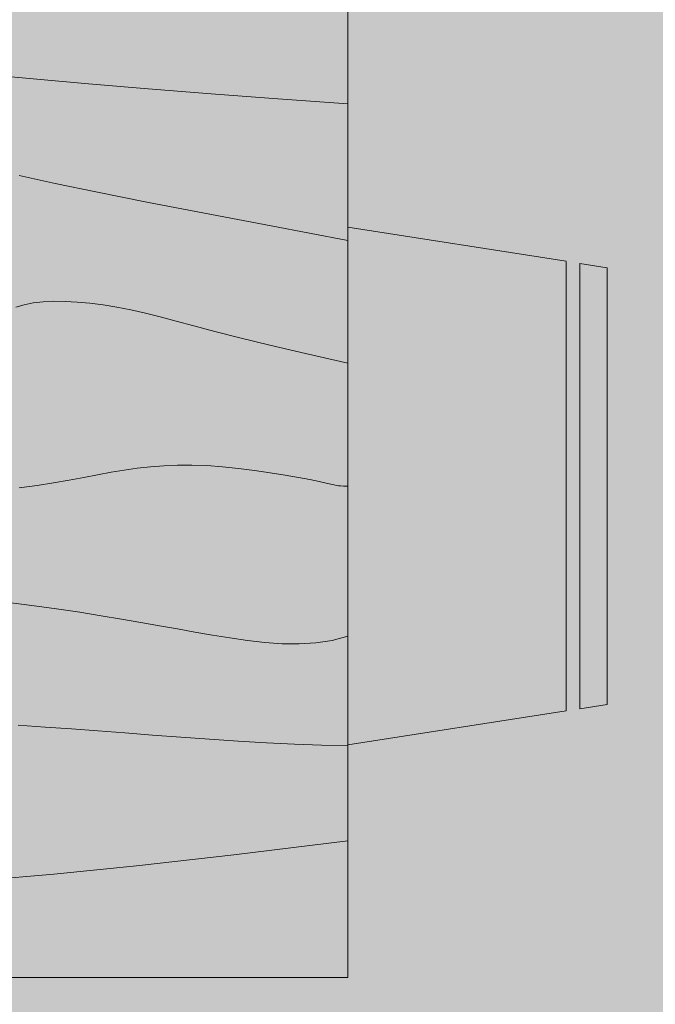
# Model space of a CAD drawing. Units: inches. Extents: x 3024 to 3952, y 1308 to 1863.
# Tile 11 of 29: x 3374 to 3392, y 1587 to 1613. Entities that reach past the tile are written whole.
import ezdxf

# ---------------------------------------------------------------- set-up
doc = ezdxf.new("R2010")
doc.units = ezdxf.units.IN
doc.layers.add('A-FLOR-PATT', color=254, linetype='Continuous', lineweight=13, true_color=0xfeeab9)
for name, color, linetype, lineweight in [('A-FLOR-TILE-PATT', 7, 'Continuous', 13), ('A-FURN', 8, 'Continuous', 18), ('A-FURN-PATT', 9, 'Continuous', 13)]:
    doc.layers.add(name, color=color, linetype=linetype, lineweight=lineweight)

# ---------------------------------------------------------------- blocks, each defined once
blk = doc.blocks.new('Dining Set - 36 x 72 in.')
for p, q in [((36, -18), (36, 18)), ((44.0006, 8.23428), (35.9976, 9.48474)), ((44, 8.23041), (44, -8.23915)), ((44.5, -8.15843), (44.5, 8.15338)), ((45.5, 8), (44.5005, 8.15617)), ((45.5, 8), (45.5, -8)), ((35.9976, -9.48476), (43.9993, -8.2345)), ((44.4997, -8.15631), (45.5, -8)), ((-36, -18), (36, -18))]:
    blk.add_line(p, q)
for points in [[(22.5879, 15.08984), (24.4721, 14.91715), (26.5052, 14.73958), (28.6809, 14.5581), (30.9929, 14.3737), (33.4347, 14.18733), (36, 14)], [(23.959, 11.37304), (25.2786, 11.08618), (26.8282, 10.76562), (28.6414, 10.40405), (30.752, 9.99414), (33.1936, 9.52856), (36, 9)], [(23.8358, 6.55957), (24.142, 6.64323), (24.4735, 6.70735), (24.8334, 6.75), (25.2235, 6.76969), (25.642, 6.76692), (26.0858, 6.74267), (26.5521, 6.69791), (27.0379, 6.63362), (27.5404, 6.55078), (28.0565, 6.45036), (28.5834, 6.33333), (29.1242, 6.19987), (29.7071, 6.04687), (30.3661, 5.87044), (31.1354, 5.66666), (32.0493, 5.43164), (33.142, 5.16146), (34.4475, 4.85221), (36, 4.5)], [(23.9549, -0.06836), (24.6146, 0.02083), (25.2235, 0.11784), (25.7904, 0.21875), (26.3241, 0.31966), (26.8334, 0.41666), (27.3265, 0.50618), (27.8099, 0.58593), (28.2894, 0.65397), (28.7709, 0.70833), (29.2601, 0.74707), (29.763, 0.76823), (30.2855, 0.76985), (30.8334, 0.75), (31.4088, 0.70784), (31.9994, 0.64713), (32.589, 0.57275), (33.1615, 0.48958), (33.7008, 0.4025), (34.1908, 0.3164), (34.6153, 0.23616), (34.9584, 0.16666), (35.2099, 0.11165), (35.3848, 0.07031), (35.504, 0.04069), (35.5886, 0.02083), (35.6594, 0.00879), (35.7377, 0.0026), (35.8442, 0.00032), (36, 0)], [(23.4727, -4.25391), (24.4289, -4.37549), (25.3334, -4.5), (26.1785, -4.62492), (26.9694, -4.74935), (27.7145, -4.87281), (28.4219, -4.99479), (29.1, -5.11483), (29.7572, -5.23242), (30.4016, -5.34709), (31.0417, -5.45834), (31.6837, -5.56437), (32.3262, -5.65821), (32.9658, -5.73153), (33.599, -5.77604), (34.2224, -5.78345), (34.8327, -5.74545), (35.4264, -5.65373), (36, -5.5)], [(23.9271, -8.76563), (24.9081, -8.82707), (25.8763, -8.89388), (26.8465, -8.96558), (27.8334, -9.04167), (28.8474, -9.12118), (29.8828, -9.20117), (30.93, -9.27824), (31.9792, -9.34896), (33.0205, -9.40991), (34.0443, -9.45768), (35.0407, -9.48885), (36, -9.5)], [(0.2448, -14.26042), (1.7647, -14.3169), (3.1973, -14.3763), (4.5507, -14.43767), (5.8333, -14.5), (7.0554, -14.5621), (8.235, -14.62175), (9.3922, -14.67652), (10.5469, -14.72396), (11.7192, -14.76164), (12.929, -14.78711), (14.1965, -14.79794), (15.5417, -14.79167), (16.9933, -14.76424), (18.6152, -14.70508), (20.4804, -14.60197), (22.6615, -14.44271), (25.2312, -14.21509), (28.2624, -13.9069), (31.8277, -13.50594), (36, -13)]]:
    blk.add_lwpolyline(points)

msp = doc.modelspace()

# ---------------------------------------------------------------- hatches: boundary and pattern name
at = {"layer": 'A-FLOR-PATT', "transparency": 33554528}
h = msp.add_hatch(color=256, dxfattribs=at)
h.dxf.hatch_style = 1
h.paths.add_polyline_path([(3460.764, 1688.6064), (3412.764, 1688.6064), (3412.764, 1694.6064), (3460.764, 1694.6064), (3460.764, 1778.6064), (3406.764, 1778.6064), (3406.764, 1759.9514), (3318.2981, 1759.9514), (3318.2981, 1658.6064), (3322.5356, 1658.6064), (3322.5356, 1652.6064), (3292.764, 1652.6064), (3292.764, 1778.6064), (3106.764, 1778.6064), (3106.764, 1628.6064), (3172.764, 1628.6064), (3172.764, 1532.6064), (3166.764, 1532.6064), (3166.764, 1628.6064), (3106.764, 1628.6064), (3106.764, 1356.8452), (3202.812, 1356.8452), (3202.812, 1354.2534), (3202.812, 1353.8388), (3202.812, 1351.1212), (3202.812, 1347.8452), (3277.764, 1347.8452), (3277.764, 1353.8452), (3277.764, 1356.8452), (3277.764, 1442.6064), (3460.764, 1442.6064)])
h.paths.add_polyline_path([(3216.238, 1527.2064), (3216.238, 1491.2064), (3214.663, 1491.2064), (3214.663, 1491.2409, -0.3966224), (3180.243, 1526.6064), (3163.0285, 1526.6064), (3163.0285, 1531.1064), (3161.716, 1531.1064), (3161.716, 1561.1064), (3163.0285, 1561.1064), (3163.0285, 1531.1064), (3163.0285, 1526.6064), (3180.243, 1526.6064, 0.3966224), (3214.663, 1491.2409), (3214.663, 1527.2064)], flags=16)
h.paths.add_polyline_path([(3227.364, 1649.8972), (3191.364, 1649.8972), (3191.364, 1651.4722), (3227.364, 1651.4722)], flags=16)
h.paths.add_polyline_path([(3323.1172, 1606.7362), (3323.8545, 1606.8514), (3323.8545, 1594.8241), (3323.1172, 1594.9393)], flags=16)
h.paths.add_polyline_path([(3324.2232, 1606.909), (3330.1216, 1607.8307), (3330.1216, 1614.1093), (3339.3495, 1614.1093), (3340.2711, 1620.0078), (3352.4136, 1620.0078), (3353.3353, 1614.1093), (3359.9941, 1614.1093), (3360.9157, 1620.0078), (3373.0582, 1620.0078), (3373.9799, 1614.1093), (3383.2077, 1614.1093), (3383.2077, 1607.8307), (3389.1062, 1606.909), (3389.1062, 1594.7665), (3383.2077, 1593.8449), (3383.2077, 1587.5663), (3373.9799, 1587.5663), (3373.0583, 1581.6678), (3360.9157, 1581.6678), (3359.9941, 1587.5663), (3353.3353, 1587.5663), (3352.4136, 1581.6678), (3340.2711, 1581.6678), (3339.3495, 1587.5663), (3330.1216, 1587.5663), (3330.1216, 1593.8449), (3324.2232, 1594.7665)], flags=16)
h.paths.add_polyline_path([(3236.1584, 1693.1064), (3236.1584, 1723.1064), (3237.4709, 1723.1064), (3237.4709, 1693.1064)], flags=16)
h.paths.add_polyline_path([(3373.2158, 1600.6847), (3373.7965, 1600.7303), (3374.3268, 1600.7874), (3374.8132, 1600.8531), (3375.2621, 1600.9247), (3375.6801, 1600.9991), (3376.0736, 1601.0735), (3376.6855, 1601.19), (3377.366, 1601.3023), (3378.0667, 1601.3814), (3378.8026, 1601.4123), (3379.5865, 1601.3839), (3380.4537, 1601.2948), (3381.301, 1601.1717), (3382.0317, 1601.0433), (3382.4398, 1600.9607), (3382.6252, 1600.9201), (3382.919, 1600.8507), (3382.9044, 1600.8531), (3382.842, 1600.8678), (3382.7541, 1600.8896), (3382.6252, 1600.9201), (3382.4398, 1600.9607), (3382.1868, 1601.0119), (3381.8738, 1601.0711), (3381.5125, 1601.1346), (3381.1149, 1601.1988), (3380.6928, 1601.2601), (3380.2581, 1601.3149), (3379.8226, 1601.3597), (3379.3984, 1601.3908), (3378.9944, 1601.4054), (3378.6092, 1601.4042), (3378.2384, 1601.3886), (3377.8777, 1601.36), (3377.5227, 1601.32), (3377.1691, 1601.2698), (3376.8127, 1601.211), (3376.4491, 1601.145), (3376.0736, 1601.0735), (3375.4177, 1600.9494), (3374.5542, 1600.8119), (3373.5044, 1600.6988)], flags=0)
h.paths.add_polyline_path([(3380.0253, 1596.7351), (3380.499, 1596.6659), (3380.9706, 1596.6119), (3381.4375, 1596.5791), (3381.8971, 1596.5736), (3382.5886, 1596.6167), (3382.7848, 1596.6692), (3382.1465, 1596.5706), (3381.236, 1596.5815), (3380.3199, 1596.6865)], flags=0)
h.paths.add_polyline_path([(3369.6414, 1603.9617), (3370.1589, 1604.0021), (3370.6218, 1604.0539), (3371.0335, 1604.1173), (3371.3978, 1604.1921), (3371.7181, 1604.2785), (3371.9984, 1604.3761), (3372.2441, 1604.483), (3372.4611, 1604.5972), (3372.655, 1604.7163), (3372.8317, 1604.8384), (3372.9968, 1604.9611), (3373.3703, 1605.2455), (3373.8426, 1605.5328), (3374.4624, 1605.7539), (3375.1058, 1605.8302), (3375.7221, 1605.8261), (3376.4109, 1605.76), (3377.1534, 1605.6376), (3377.8945, 1605.473), (3378.1382, 1605.409), (3377.7394, 1605.5074), (3377.3509, 1605.5937), (3376.9704, 1605.6677), (3376.5999, 1605.7288), (3376.2417, 1605.7762), (3375.8979, 1605.8092), (3375.5707, 1605.8271), (3375.2621, 1605.8291), (3374.9745, 1605.8146), (3374.7092, 1605.7832), (3374.4647, 1605.7359), (3374.239, 1605.6742), (3374.0298, 1605.5996), (3373.835, 1605.5134), (3373.6525, 1605.4171), (3373.4801, 1605.3123), (3373.3156, 1605.2002), (3373.1562, 1605.0825), (3372.7603, 1604.781), (3372.236, 1604.4588), (3371.5738, 1604.2283), (3370.8493, 1604.0794), (3369.9262, 1603.976)], flags=0)
h.paths.add_polyline_path([(3366.7533, 1606.5832), (3367.1713, 1606.5519), (3367.5378, 1606.5374), (3367.8568, 1606.5394), (3368.1325, 1606.5573), (3368.3694, 1606.5903), (3368.5717, 1606.6377), (3368.7438, 1606.6988), (3368.89, 1606.7728), (3369.0146, 1606.8591), (3369.121, 1606.9568), (3369.2094, 1607.0646), (3369.2792, 1607.181), (3369.3295, 1607.3046), (3369.3596, 1607.4339), (3369.3688, 1607.5676), (3369.3565, 1607.7042), (3369.3218, 1607.8422), (3369.2649, 1607.9804), (3369.1893, 1608.1187), (3369.0993, 1608.2569), (3368.9992, 1608.3952), (3368.8934, 1608.5334), (3368.7861, 1608.6717), (3368.6817, 1608.8099), (3368.4212, 1609.1804), (3368.2685, 1609.7106), (3368.4883, 1610.1814), (3369.0537, 1610.4604), (3369.6717, 1610.5097), (3370.2812, 1610.3612), (3370.4805, 1610.2968), (3370.1882, 1610.3839), (3369.9284, 1610.4472), (3369.6905, 1610.4842), (3369.4662, 1610.4933), (3369.2555, 1610.4765), (3369.0608, 1610.4367), (3368.884, 1610.3767), (3368.7274, 1610.2994), (3368.5931, 1610.2077), (3368.4833, 1610.1045), (3368.4002, 1609.9927), (3368.3451, 1609.8747), (3368.3166, 1609.7517), (3368.3127, 1609.6244), (3368.331, 1609.4935), (3368.3696, 1609.3597), (3368.4261, 1609.2237), (3368.4985, 1609.0863), (3368.5845, 1608.9482), (3368.6817, 1608.8099), (3368.7861, 1608.6717), (3368.8934, 1608.5334), (3368.9992, 1608.3952), (3369.0993, 1608.2569), (3369.3398, 1607.8876), (3369.3941, 1607.2896), (3368.9774, 1606.7817), (3368.3928, 1606.5742), (3367.7162, 1606.5303), (3367.0044, 1606.5585)], flags=0)
h.paths.add_polyline_path([(3362.1859, 1610.2589), (3362.5478, 1610.2845), (3362.8348, 1610.3275), (3363.0585, 1610.3863), (3363.2303, 1610.4595), (3363.3619, 1610.5457), (3363.463, 1610.6432), (3363.5376, 1610.7502), (3363.5876, 1610.8643), (3363.6153, 1610.9834), (3363.6229, 1611.1055), (3363.6125, 1611.2283), (3363.5861, 1611.3496), (3363.5462, 1611.4673), (3363.4949, 1611.5797), (3363.4358, 1611.6871), (3363.3723, 1611.7902), (3363.3081, 1611.8897), (3363.2468, 1611.9863), (3363.192, 1612.0808), (3363.0258, 1612.4261), (3363.3371, 1612.8672), (3363.9008, 1612.9782), (3364.4822, 1612.9641), (3365.1098, 1612.9074), (3365.328, 1612.8805), (3364.9615, 1612.9208), (3364.6426, 1612.9496), (3364.3668, 1612.9669), (3364.1299, 1612.9726), (3363.9276, 1612.9669), (3363.7555, 1612.9496), (3363.6093, 1612.9208), (3363.4848, 1612.8805), (3363.3782, 1612.8289), (3363.2889, 1612.7672), (3363.2169, 1612.6969), (3363.1622, 1612.6193), (3363.1247, 1612.5361), (3363.1046, 1612.4484), (3363.1017, 1612.358), (3363.1161, 1612.266), (3363.1472, 1612.1738), (3363.192, 1612.0808), (3363.2468, 1611.9863), (3363.3081, 1611.8897), (3363.3723, 1611.7902), (3363.4358, 1611.6871), (3363.6363, 1611.323), (3363.5979, 1610.7003), (3363.0863, 1610.3651), (3362.3983, 1610.2622)], flags=0)
h.paths.add_polyline_path([(3352.356, 1581.2991), (3352.2408, 1580.5618), (3340.4439, 1580.5618), (3340.3287, 1581.2991)], flags=16)
h.paths.add_polyline_path([(3340.4439, 1621.1137), (3352.2408, 1621.1137), (3352.356, 1620.3764), (3340.3287, 1620.3764)], flags=16)
h.paths.add_polyline_path([(3278.4282, 1504.7424), (3290.3831, 1504.7424), (3290.3831, 1502.7499), (3291.0473, 1502.7499), (3291.0473, 1494.7799), (3290.3831, 1494.7799), (3290.3831, 1494.1158), (3291.0473, 1494.1158), (3291.0473, 1486.1458), (3290.3831, 1486.1458), (3290.3831, 1484.1533), (3291.0473, 1484.1533), (3291.0473, 1483.4892, -0.0909091), (3291.0473, 1468.8776), (3291.0473, 1468.2135), (3290.3831, 1468.2135), (3290.3831, 1464.8926), (3278.4282, 1464.8926), (3278.4282, 1472.8626), (3277.764, 1473.5268), (3277.764, 1478.84), (3278.4282, 1479.5042)], flags=16)
h.paths.add_polyline_path([(3278.7603, 1504.4103), (3290.051, 1504.4103), (3290.051, 1465.2247), (3278.7603, 1465.2247)], flags=0)
h.paths.add_polyline_path([(3123.904, 1600.7821), (3117.9039, 1602.7821), (3117.9039, 1599.7821), (3119.4039, 1599.7821), (3119.4039, 1596.7821), (3118.4039, 1596.7821), (3118.4039, 1598.7821), (3117.9039, 1598.7821), (3117.9039, 1596.2821), (3109.9039, 1596.2821), (3109.9039, 1617.2821), (3117.9039, 1617.2821), (3117.9039, 1610.7821), (3123.9038, 1612.7821, -0.7025712), (3137.9039, 1606.7822, -0.7025621)], flags=16)
h.paths.add_polyline_path([(3123.9039, 1602.7822), (3123.9039, 1610.7822, -0.7345333), (3136.9039, 1606.7822, -0.7345297)], flags=0)
h.paths.add_polyline_path([(3177.972, 1689.6473), (3109.2405, 1689.6473), (3109.2405, 1741.1959), (3177.972, 1741.1959)], flags=16)
h.paths.add_polyline_path([(3373.0006, 1581.2991), (3372.8854, 1580.5618), (3361.0885, 1580.5618), (3360.9733, 1581.2991)], flags=16)
h.paths.add_polyline_path([(3361.0885, 1621.1137), (3372.8854, 1621.1137), (3373.0006, 1620.3764), (3360.9733, 1620.3764)], flags=16)
h.paths.add_polyline_path([(3116.9039, 1598.2821, -0.4142136), (3116.1539, 1597.2821), (3111.9039, 1597.2821, -0.4142136), (3110.9039, 1598.0321), (3110.9039, 1615.2821, -0.4142136), (3111.6539, 1616.2821), (3115.9039, 1616.2821, -0.4142136), (3116.9039, 1615.5321)], flags=0)
h.paths.add_polyline_path([(3121.6122, 1728.1369), (3121.6122, 1696.5205), (3110.2715, 1696.5205), (3110.2715, 1714.3906), (3121.6122, 1714.3906), (3121.6122, 1716.4526), (3110.2715, 1716.4526), (3110.2715, 1734.3228), (3123.3304, 1734.3228), (3123.3304, 1729.8552), (3134.6711, 1741.1959), (3134.6711, 1728.1369)], flags=0)
h.paths.add_polyline_path([(3389.4748, 1606.8514), (3390.2122, 1606.7362), (3390.2122, 1594.9393), (3389.4748, 1594.8241)], flags=16)
h.paths.add_polyline_path([(3257.6842, 1762.8281), (3259.6842, 1768.8281), (3256.6842, 1768.8281), (3256.6842, 1767.3281), (3253.6842, 1767.3281), (3253.6842, 1768.3281), (3255.6842, 1768.3281), (3255.6842, 1768.8281), (3253.1842, 1768.8281), (3253.1842, 1776.8281), (3274.1842, 1776.8281), (3274.1842, 1768.8281), (3267.6842, 1768.8281), (3269.6842, 1762.8282, -0.7025712), (3263.6843, 1748.8282, -0.7025621)], flags=16)
h.paths.add_polyline_path([(3259.6842, 1762.8281), (3267.6843, 1762.8281, -0.7345333), (3263.6842, 1749.8282, -0.7345297)], flags=0)
h.paths.add_polyline_path([(3411.264, 1715.6064), (3411.264, 1716.9189), (3441.264, 1716.9189), (3441.264, 1715.6064)], flags=16)
h.paths.add_polyline_path([(3178.3806, 1449.1876), (3178.3806, 1397.639), (3109.6491, 1397.639), (3109.6491, 1449.1876)], flags=16)
h.paths.add_polyline_path([(3397.1501, 1541.7146), (3419.6183, 1541.7146), (3419.6183, 1496.7783), (3397.1501, 1496.7783)], flags=16)
h.paths.add_polyline_path([(3254.1842, 1770.5781), (3254.1842, 1774.8281, -0.4142136), (3254.9342, 1775.8281), (3272.1842, 1775.8281, -0.4142136), (3273.1842, 1775.0781), (3273.1842, 1770.8281, -0.4142136), (3272.4342, 1769.8281), (3255.1842, 1769.8281, -0.4142136)], flags=0)
h.paths.add_polyline_path([(3403.672, 1500.7601), (3403.6016, 1500.3997), (3403.5328, 1500.0441), (3403.4662, 1499.6867), (3403.4027, 1499.3226), (3403.3464, 1498.9532), (3403.3025, 1498.5811), (3403.2759, 1498.2091), (3403.2714, 1497.8401), (3403.3064, 1497.2813), (3403.3491, 1497.1219), (3403.2689, 1497.6395), (3403.2778, 1498.3719), (3403.3635, 1499.0984), (3403.4889, 1499.8168), (3403.6016, 1500.3997), (3403.672, 1500.7601), (3403.744, 1501.1315), (3403.817, 1501.5205), (3403.891, 1501.9336), (3403.9656, 1502.3769), (3404.0404, 1502.8572), (3404.115, 1503.3786), (3404.2264, 1504.2311), (3404.2571, 1504.5223), (3404.1552, 1503.6598), (3404.0063, 1502.6193), (3403.8604, 1501.7518), (3403.744, 1501.1315)], flags=0)
h.paths.add_polyline_path([(3406.5868, 1505.0416), (3406.6121, 1504.5236), (3406.6492, 1504.0526), (3406.6956, 1503.624), (3406.7491, 1503.2333), (3406.8072, 1502.8759), (3406.8676, 1502.5473), (3406.9281, 1502.243), (3407.0268, 1501.7597), (3407.1416, 1501.1368), (3407.2087, 1500.3904), (3407.1804, 1499.6703), (3407.1078, 1498.9956), (3407.0074, 1498.3199), (3406.8809, 1497.6059), (3406.7403, 1496.9627), (3406.7418, 1496.9824), (3406.7491, 1497.0249), (3406.8229, 1497.3409), (3406.8364, 1497.4025), (3406.878, 1497.6078), (3406.9261, 1497.8614), (3406.9777, 1498.1526), (3407.0298, 1498.4712), (3407.0797, 1498.8068), (3407.1243, 1499.149), (3407.1607, 1499.4874), (3407.1859, 1499.8115), (3407.1978, 1500.1137), (3407.1969, 1500.3962), (3407.1841, 1500.6642), (3407.1609, 1500.9225), (3407.1284, 1501.1761), (3407.0876, 1501.43), (3407.0398, 1501.6891), (3406.9862, 1501.9585), (3406.8832, 1502.4628), (3406.7712, 1503.0713), (3406.6657, 1503.8424), (3406.5924, 1504.7735)], flags=0)
h.paths.add_polyline_path([(3409.2517, 1507.8962), (3409.2752, 1507.4282), (3409.3079, 1507.0076), (3409.3501, 1506.6314), (3409.4015, 1506.2969), (3409.4624, 1506.0009), (3409.5326, 1505.7406), (3409.6119, 1505.5128), (3409.6988, 1505.3131), (3409.7915, 1505.1368), (3409.8883, 1504.9792), (3409.9875, 1504.8356), (3410.0872, 1504.7015), (3410.1859, 1504.572), (3410.4508, 1504.2132), (3410.7205, 1503.6035), (3410.8059, 1502.8824), (3410.7619, 1502.0875), (3410.6122, 1501.2299), (3410.4402, 1500.6169), (3410.2538, 1500.0031), (3410.0536, 1499.3219), (3409.9909, 1499.0812), (3410.1761, 1499.7472), (3410.3596, 1500.3513), (3410.4512, 1500.6561), (3410.5312, 1500.9412), (3410.6013, 1501.226), (3410.6614, 1501.512), (3410.7111, 1501.7964), (3410.7496, 1502.0763), (3410.7764, 1502.3489), (3410.7909, 1502.6114), (3410.7926, 1502.8608), (3410.7808, 1503.0944), (3410.7553, 1503.31), (3410.7169, 1503.5087), (3410.6667, 1503.6921), (3410.6061, 1503.8621), (3410.5361, 1504.0203), (3410.4578, 1504.1686), (3410.3726, 1504.3088), (3410.2815, 1504.4424), (3410.1859, 1504.572), (3410.0872, 1504.7015), (3409.859, 1505.0083), (3409.5943, 1505.5117), (3409.4266, 1506.1336), (3409.324, 1506.8011), (3409.2586, 1507.6407)], flags=0)
h.paths.add_polyline_path([(3411.4914, 1510.5878), (3411.4432, 1510.1586), (3411.4054, 1509.775), (3411.38, 1509.4354), (3411.3681, 1509.1376), (3411.3698, 1508.8784), (3411.3843, 1508.6542), (3411.4112, 1508.4618), (3411.4497, 1508.2974), (3411.4994, 1508.1575), (3411.5595, 1508.0388), (3411.6296, 1507.9375), (3411.7097, 1507.851), (3411.802, 1507.7792), (3411.9096, 1507.7225), (3412.0353, 1507.6817), (3412.1821, 1507.6572), (3412.3528, 1507.6496), (3412.5505, 1507.6597), (3412.778, 1507.6879), (3413.0364, 1507.7341), (3413.3194, 1507.7955), (3413.6188, 1507.8687), (3413.9264, 1507.95), (3414.234, 1508.036), (3414.5333, 1508.1232), (3414.8163, 1508.208), (3415.0747, 1508.287), (3415.3023, 1508.3569), (3415.5007, 1508.4158), (3415.6733, 1508.4617), (3416.1158, 1508.5538), (3416.512, 1508.2591), (3416.716, 1507.6581), (3416.61, 1507.0003), (3416.3052, 1506.3411), (3415.8928, 1505.618), (3415.7339, 1505.3633), (3415.9914, 1505.791), (3416.201, 1506.1583), (3416.3666, 1506.4739), (3416.4925, 1506.7462), (3416.5828, 1506.9838), (3416.6413, 1507.1949), (3416.6725, 1507.3883), (3416.6799, 1507.5705), (3416.6662, 1507.7417), (3416.6339, 1507.9), (3416.5851, 1508.0436), (3416.5223, 1508.1709), (3416.4478, 1508.28), (3416.3639, 1508.3692), (3416.273, 1508.4368), (3416.1765, 1508.4815), (3416.0718, 1508.5047), (3415.9553, 1508.5079), (3415.8237, 1508.493), (3415.6733, 1508.4617), (3415.5007, 1508.4158), (3415.3327, 1508.3659), (3414.6495, 1508.157), (3414.0606, 1507.9855), (3413.4456, 1507.8229), (3412.8838, 1507.701), (3412.5505, 1507.6597), (3412.0748, 1507.6354), (3411.595, 1507.8883), (3411.398, 1508.4429), (3411.3624, 1508.9927), (3411.3854, 1509.5711), (3411.4578, 1510.3071)], flags=0)
h.paths.add_polyline_path([(3135.0797, 1449.1876), (3135.0797, 1436.1286), (3122.0208, 1436.1286), (3122.0208, 1404.5122), (3110.6801, 1404.5122), (3110.6801, 1422.3823), (3122.0208, 1422.3823), (3122.0208, 1424.4443), (3110.6801, 1424.4443), (3110.6801, 1442.3145), (3123.739, 1442.3145), (3123.739, 1437.8469)], flags=0)
h.paths.add_polyline_path([(3416.4944, 1514.2949), (3416.4837, 1513.8511), (3416.4893, 1513.4867), (3416.5102, 1513.1926), (3416.5451, 1512.9593), (3416.5929, 1512.7775), (3416.6524, 1512.6379), (3416.7224, 1512.531), (3416.8017, 1512.4488), (3416.8886, 1512.3882), (3416.9813, 1512.3476), (3417.0781, 1512.3251), (3417.1773, 1512.3189), (3417.277, 1512.3274), (3417.3757, 1512.3488), (3417.4713, 1512.3813), (3417.5627, 1512.4229), (3417.65, 1512.471), (3417.7338, 1512.5225), (3417.8146, 1512.5747), (3417.8931, 1512.6245), (3417.9699, 1512.6691), (3418.2968, 1512.8265), (3418.6505, 1512.4645), (3418.7037, 1511.9342), (3418.6693, 1511.3839), (3418.6076, 1510.8228), (3418.5777, 1510.5927), (3418.6197, 1510.9333), (3418.6525, 1511.2311), (3418.6759, 1511.4903), (3418.6899, 1511.7144), (3418.6946, 1511.9069), (3418.6899, 1512.0713), (3418.6759, 1512.2112), (3418.6525, 1512.33), (3418.6197, 1512.4311), (3418.5778, 1512.5177), (3418.5276, 1512.5903), (3418.4705, 1512.6488), (3418.4075, 1512.6933), (3418.3399, 1512.7237), (3418.2686, 1512.7401), (3418.1951, 1512.7424), (3418.1204, 1512.7307), (3418.0455, 1512.7055), (3417.9792, 1512.6736), (3417.65, 1512.471), (3417.5627, 1512.4229), (3417.4713, 1512.3813), (3417.3757, 1512.3488), (3417.277, 1512.3274), (3416.878, 1512.2936), (3416.5757, 1512.7549), (3416.492, 1513.3145), (3416.4808, 1514.0384)], flags=0)
h.paths.add_polyline_path([(3392.8223, 1481.9454), (3396.7707, 1481.9454), (3396.7707, 1480.9201), (3428.3585, 1480.9201), (3428.3585, 1481.9454), (3432.3069, 1481.9454), (3432.3069, 1464.8354, -0.266667), (3392.8223, 1464.8354)], flags=16)
h.paths.add_polyline_path([(3431.203, 1547.5428), (3450.8613, 1547.5428, -0.1904762), (3450.8614, 1484.031), (3431.203, 1484.031), (3431.203, 1488.5675), (3432.3809, 1488.5675), (3432.3809, 1543.0062), (3431.203, 1543.0062)], flags=16)
h.paths.add_polyline_path([(3451.9233, 1524.86, -0.0496282), (3451.9233, 1506.7138), (3446.7921, 1506.7138), (3446.7921, 1524.86)], flags=0)
h.paths.add_polyline_path([(3460.764, 1436.6064), (3277.764, 1436.6064), (3277.764, 1356.8452), (3277.764, 1353.8452), (3460.764, 1353.8452)], flags=17)
h.paths.add_polyline_path([(3121.3033, 1577.378), (3153.693, 1577.378), (3153.693, 1586.6752), (3121.3033, 1586.6752)], flags=24)
h.paths.add_polyline_path([(3164.1457, 1464.1276), (3210.4801, 1464.1276), (3210.4801, 1473.4247), (3164.1457, 1473.4247)], flags=24)
h.paths.add_polyline_path([(3343.1909, 1505.8863), (3373.7236, 1505.8863), (3373.7236, 1515.1773), (3343.1909, 1515.1773)], flags=24)
h.paths.add_polyline_path([(3337.6353, 1564.2926), (3370.0189, 1564.2926), (3370.0189, 1573.5836), (3337.6353, 1573.5836)], flags=24)
h.paths.add_polyline_path([(3419.204, 1753.8578), (3453.3997, 1753.8578), (3453.3997, 1762.9956), (3419.204, 1762.9956)], flags=24)
h.paths.add_polyline_path([(3341.2523, 1701.0246), (3381.0761, 1701.0246), (3381.0761, 1710.3156), (3341.2523, 1710.3156)], flags=24)
h.paths.add_polyline_path([(3245.8895, 1726.2997), (3278.2793, 1726.2997), (3278.2793, 1735.5968), (3245.8895, 1735.5968)], flags=24)
h.paths.add_polyline_path([(3128.8045, 1668.6736), (3175.1389, 1668.6736), (3175.1389, 1677.9707), (3128.8045, 1677.9707)], flags=24)
h.paths.add_polyline_path([(3345.9997, 1396.0062), (3389.09, 1396.0062), (3389.09, 1405.3033), (3345.9997, 1405.3033)], flags=24)
at = {"layer": 'A-FLOR-TILE-PATT', "transparency": 33554569}
h = msp.add_hatch(dxfattribs=at)
h.set_pattern_fill('ANGLE', color=256, scale=2)
h.set_pattern_definition([(0, (0, 0), (0, 13.97), [10.16, -3.81]), (90, (0, 0), (-13.97, 9e-16), [10.16, -3.81])])
h.paths.add_polyline_path([(3292.764, 1778.6064), (3232.764, 1778.6064), (3232.764, 1694.6064), (3236.1584, 1694.6064), (3236.1584, 1723.1064), (3237.4709, 1723.1064), (3237.4709, 1723.0777, -0.3870039), (3266.1209, 1694.6064), (3292.764, 1694.6064)])
h.paths.add_polyline_path([(3263.6843, 1748.8282, -0.7025621), (3257.6842, 1762.8281), (3259.6842, 1768.8281), (3256.6842, 1768.8281), (3256.6842, 1767.3281), (3253.6842, 1767.3281), (3253.6842, 1768.3281), (3255.6842, 1768.3281), (3255.6842, 1768.8281), (3253.1842, 1768.8281), (3253.1842, 1776.8281), (3274.1842, 1776.8281), (3274.1842, 1768.8281), (3267.6842, 1768.8281), (3269.6842, 1762.8282, -0.7025712)], flags=16)
h.paths.add_polyline_path([(3263.6842, 1749.8282, -0.7345297), (3259.6842, 1762.8281), (3267.6843, 1762.8281, -0.7345333)], flags=0)
h.paths.add_polyline_path([(3255.1842, 1769.8281, -0.4142136), (3254.1842, 1770.5781), (3254.1842, 1774.8281, -0.4142136), (3254.9342, 1775.8281), (3272.1842, 1775.8281, -0.4142136), (3273.1842, 1775.0781), (3273.1842, 1770.8281, -0.4142136), (3272.4342, 1769.8281)], flags=0)
h.paths.add_polyline_path([(3460.764, 1436.6064), (3277.764, 1436.6064), (3277.764, 1356.8452), (3277.764, 1353.8452), (3460.764, 1353.8452)])
h.paths.add_polyline_path([(3166.764, 1628.6064), (3106.764, 1628.6064), (3106.764, 1532.6064), (3133.066, 1532.6064, -0.3870039), (3161.716, 1561.0777), (3161.716, 1561.1064), (3163.0285, 1561.1064), (3163.0285, 1532.6064), (3166.764, 1532.6064)])
h.paths.add_polyline_path([(3123.904, 1600.7821), (3117.9039, 1602.7821), (3117.9039, 1599.7821), (3119.4039, 1599.7821), (3119.4039, 1596.7821), (3118.4039, 1596.7821), (3118.4039, 1598.7821), (3117.9039, 1598.7821), (3117.9039, 1596.2821), (3109.9039, 1596.2821), (3109.9039, 1617.2821), (3117.9039, 1617.2821), (3117.9039, 1610.7821), (3123.9038, 1612.7821, -0.7025712), (3137.9039, 1606.7822, -0.7025621)], flags=16)
h.paths.add_polyline_path([(3123.9039, 1602.7822), (3123.9039, 1610.7822, -0.7345333), (3136.9039, 1606.7822, -0.7345297)], flags=0)
h.paths.add_polyline_path([(3116.1539, 1597.2821), (3111.9039, 1597.2821, -0.4142136), (3110.9039, 1598.0321), (3110.9039, 1615.2821, -0.4142136), (3111.6539, 1616.2821), (3115.9039, 1616.2821, -0.4142136), (3116.9039, 1615.5321), (3116.9039, 1598.2821, -0.4142136)], flags=0)
h.paths.add_polyline_path([(3245.8895, 1726.2997), (3278.2793, 1726.2997), (3278.2793, 1735.5968), (3245.8895, 1735.5968)], flags=24)
h.paths.add_polyline_path([(3345.9997, 1396.0062), (3389.09, 1396.0062), (3389.09, 1405.3033), (3345.9997, 1405.3033)], flags=24)
h.paths.add_polyline_path([(3121.3033, 1577.378), (3153.693, 1577.378), (3153.693, 1586.6752), (3121.3033, 1586.6752)], flags=24)
at = {"layer": 'A-FURN-PATT', "transparency": 33554511}
h = msp.add_hatch(color=256, dxfattribs=at)
h.dxf.hatch_style = 1
h.paths.add_polyline_path([(3373.0582, 1620.0078), (3360.9157, 1620.0078), (3359.9941, 1614.1093), (3373.9799, 1614.1093)])
h.paths.add_polyline_path([(3372.8854, 1621.1137), (3361.0885, 1621.1137), (3360.9733, 1620.3764), (3373.0006, 1620.3764)])
h.paths.add_polyline_path([(3389.1062, 1606.909), (3383.2077, 1607.8307), (3383.2077, 1593.8449), (3389.1062, 1594.7665)])
h.paths.add_polyline_path([(3390.2122, 1606.7362), (3389.4748, 1606.8514), (3389.4748, 1594.8241), (3390.2122, 1594.9393)])
h.paths.add_polyline_path([(3373.9799, 1587.5663), (3359.9941, 1587.5663), (3360.9157, 1581.6678), (3373.0583, 1581.6678)])
h.paths.add_polyline_path([(3373.0006, 1581.2991), (3360.9733, 1581.2991), (3361.0885, 1580.5618), (3372.8854, 1580.5618)])
h.paths.add_polyline_path([(3353.3353, 1587.5663), (3339.3495, 1587.5663), (3340.2711, 1581.6678), (3352.4136, 1581.6678)])
h.paths.add_polyline_path([(3352.356, 1581.2991), (3340.3287, 1581.2991), (3340.4439, 1580.5618), (3352.2408, 1580.5618)])
h.paths.add_polyline_path([(3330.1216, 1607.8307), (3324.2232, 1606.909), (3324.2232, 1594.7665), (3330.1216, 1593.8449)])
h.paths.add_polyline_path([(3323.8545, 1606.8514), (3323.1172, 1606.7362), (3323.1172, 1594.9393), (3323.8545, 1594.8241)])
h.paths.add_polyline_path([(3352.4136, 1620.0078), (3340.2711, 1620.0078), (3339.3495, 1614.1093), (3353.3353, 1614.1093)])
h.paths.add_polyline_path([(3352.2408, 1621.1137), (3340.4439, 1621.1137), (3340.3287, 1620.3764), (3352.356, 1620.3764)])
at = {"layer": 'A-FURN-PATT', "transparency": 33554600}
h = msp.add_hatch(color=256, dxfattribs=at)
h.dxf.hatch_style = 1
h.paths.add_polyline_path([(3363.5462, 1611.4673), (3363.4949, 1611.5797), (3363.4358, 1611.6871), (3363.3723, 1611.7902), (3363.2557, 1611.9708), (3363.16, 1612.1359), (3363.1003, 1612.3129), (3363.1061, 1612.4946), (3363.1815, 1612.6623), (3363.3264, 1612.8038), (3363.5397, 1612.9071), (3363.7555, 1612.9496), (3363.9276, 1612.9669), (3364.1299, 1612.9726), (3364.3668, 1612.9669), (3364.6426, 1612.9496), (3364.9615, 1612.9208), (3365.328, 1612.8805), (3365.7471, 1612.8287), (3366.2271, 1612.7662), (3366.7769, 1612.6936), (3367.4055, 1612.6117), (3368.1221, 1612.5211), (3368.9354, 1612.4225), (3369.8546, 1612.3168), (3370.8886, 1612.2046), (3372.0442, 1612.0866), (3373.3189, 1611.9636), (3374.7081, 1611.8363), (3376.2072, 1611.7054), (3377.8113, 1611.5716), (3379.516, 1611.4356), (3381.3163, 1611.2982), (3383.2077, 1611.1601), (3383.2077, 1614.1093), (3330.1216, 1614.1093), (3330.1216, 1611.8974), (3333.6775, 1611.8808), (3336.899, 1611.834), (3339.8144, 1611.7613), (3342.4523, 1611.667), (3344.8411, 1611.5554), (3347.0091, 1611.4308), (3348.985, 1611.2976), (3350.797, 1611.1601), (3352.4691, 1611.0223), (3354.0078, 1610.8874), (3355.4146, 1610.7583), (3356.6916, 1610.6378), (3357.8403, 1610.5289), (3358.8627, 1610.4343), (3359.7605, 1610.357), (3360.5355, 1610.2999), (3361.1912, 1610.2651), (3361.7375, 1610.2519), (3362.1859, 1610.2589), (3362.5478, 1610.2845), (3362.8348, 1610.3275), (3363.0585, 1610.3863), (3363.2303, 1610.4595), (3363.3619, 1610.5457), (3363.463, 1610.6432), (3363.5376, 1610.7502), (3363.5876, 1610.8643), (3363.6153, 1610.9834), (3363.6229, 1611.1055), (3363.6125, 1611.2283), (3363.5861, 1611.3496)])
h.paths.add_polyline_path([(3368.8934, 1608.5334), (3368.7093, 1608.7706), (3368.5315, 1609.0235), (3368.3879, 1609.2961), (3368.3108, 1609.5637), (3368.3187, 1609.8182), (3368.4002, 1609.9927), (3368.4833, 1610.1045), (3368.5931, 1610.2077), (3368.7274, 1610.2994), (3368.884, 1610.3767), (3369.0608, 1610.4367), (3369.2555, 1610.4765), (3369.4662, 1610.4933), (3369.6905, 1610.4842), (3369.9284, 1610.4472), (3370.1882, 1610.3839), (3370.4805, 1610.2968), (3370.8156, 1610.1885), (3371.204, 1610.0615), (3371.6561, 1609.9183), (3372.1824, 1609.7614), (3372.7933, 1609.5933), (3373.5016, 1609.4153), (3374.3298, 1609.2232), (3375.3028, 1609.0117), (3376.4453, 1608.7754), (3377.7822, 1608.5088), (3379.3383, 1608.2065), (3381.1386, 1607.8633), (3383.2077, 1607.4735), (3383.2077, 1611.1601), (3381.3163, 1611.2982), (3379.516, 1611.4356), (3377.8113, 1611.5716), (3376.2072, 1611.7054), (3374.7081, 1611.8363), (3373.3189, 1611.9636), (3372.0442, 1612.0866), (3370.8886, 1612.2046), (3369.8546, 1612.3168), (3368.9354, 1612.4225), (3368.1221, 1612.5211), (3367.4055, 1612.6117), (3366.7769, 1612.6936), (3366.2271, 1612.7662), (3365.7471, 1612.8287), (3365.328, 1612.8805), (3364.9615, 1612.9208), (3364.6426, 1612.9496), (3364.3668, 1612.9669), (3364.1299, 1612.9726), (3363.9276, 1612.9669), (3363.7555, 1612.9496), (3363.6093, 1612.9208), (3363.4848, 1612.8805), (3363.3782, 1612.8289), (3363.2889, 1612.7672), (3363.2169, 1612.6969), (3363.1622, 1612.6193), (3363.1247, 1612.5361), (3363.1046, 1612.4484), (3363.1017, 1612.358), (3363.1161, 1612.266), (3363.1472, 1612.1738), (3363.192, 1612.0808), (3363.2468, 1611.9863), (3363.3081, 1611.8897), (3363.4181, 1611.7194), (3363.529, 1611.5178), (3363.6075, 1611.2866), (3363.6284, 1611.0397), (3363.5728, 1610.8008), (3363.4229, 1610.5856), (3363.2303, 1610.4595), (3363.0585, 1610.3863), (3362.8348, 1610.3275), (3362.5478, 1610.2845), (3362.1859, 1610.2589), (3361.7375, 1610.2519), (3361.1912, 1610.2651), (3360.5355, 1610.2999), (3359.7605, 1610.357), (3358.8627, 1610.4343), (3357.8403, 1610.5289), (3356.6916, 1610.6378), (3355.4146, 1610.7583), (3354.0078, 1610.8874), (3352.4691, 1611.0223), (3350.797, 1611.1601), (3348.985, 1611.2976), (3347.0091, 1611.4308), (3344.8411, 1611.5554), (3342.4523, 1611.667), (3339.8144, 1611.7613), (3336.899, 1611.834), (3333.6775, 1611.8808), (3330.1216, 1611.8974), (3330.1216, 1608.2109), (3335.3, 1608.3161), (3339.5794, 1608.3616), (3343.0805, 1608.3567), (3345.9238, 1608.3107), (3348.23, 1608.2331), (3350.1196, 1608.1331), (3351.7134, 1608.0202), (3353.1317, 1607.9036), (3354.475, 1607.7912), (3355.7618, 1607.6838), (3356.9902, 1607.5807), (3358.1585, 1607.4812), (3359.2649, 1607.3846), (3360.3076, 1607.2902), (3361.2846, 1607.1972), (3362.1945, 1607.1049), (3363.0358, 1607.0131), (3363.8102, 1606.9234), (3364.5198, 1606.8381), (3365.1667, 1606.7593), (3365.7532, 1606.6891), (3366.2814, 1606.6297), (3366.7533, 1606.5832), (3367.1713, 1606.5519), (3367.5378, 1606.5374), (3367.8568, 1606.5394), (3368.1325, 1606.5573), (3368.3694, 1606.5903), (3368.5717, 1606.6377), (3368.7438, 1606.6988), (3368.89, 1606.7728), (3369.0146, 1606.8591), (3369.121, 1606.9568), (3369.2094, 1607.0646), (3369.2792, 1607.181), (3369.3295, 1607.3046), (3369.3596, 1607.4339), (3369.3688, 1607.5676), (3369.3565, 1607.7042), (3369.3218, 1607.8422), (3369.2649, 1607.9804), (3369.1893, 1608.1187), (3369.0993, 1608.2569), (3368.9992, 1608.3952)])
h.paths.add_polyline_path([(3374.239, 1605.6742), (3374.4647, 1605.7359), (3374.7092, 1605.7832), (3374.9745, 1605.8146), (3375.2621, 1605.8291), (3375.5707, 1605.8271), (3375.8979, 1605.8092), (3376.2417, 1605.7762), (3376.5999, 1605.7288), (3376.9704, 1605.6677), (3377.3509, 1605.5937), (3377.7394, 1605.5074), (3378.1382, 1605.409), (3378.5679, 1605.2962), (3379.0538, 1605.1661), (3379.621, 1605.0159), (3380.2949, 1604.8426), (3381.1005, 1604.6434), (3382.0631, 1604.4154), (3383.2077, 1604.1557), (3383.2077, 1607.4735), (3381.1386, 1607.8633), (3379.3383, 1608.2065), (3377.7822, 1608.5088), (3376.4453, 1608.7754), (3375.3028, 1609.0117), (3374.3298, 1609.2232), (3373.5016, 1609.4153), (3372.7933, 1609.5933), (3372.1824, 1609.7614), (3371.6561, 1609.9183), (3371.204, 1610.0615), (3370.8156, 1610.1885), (3370.4805, 1610.2968), (3370.1882, 1610.3839), (3369.9284, 1610.4472), (3369.6905, 1610.4842), (3369.4662, 1610.4933), (3369.2555, 1610.4765), (3369.0608, 1610.4367), (3368.884, 1610.3767), (3368.7274, 1610.2994), (3368.5931, 1610.2077), (3368.4833, 1610.1045), (3368.4002, 1609.9927), (3368.3451, 1609.8747), (3368.3166, 1609.7517), (3368.3127, 1609.6244), (3368.331, 1609.4935), (3368.3696, 1609.3597), (3368.4261, 1609.2237), (3368.4985, 1609.0863), (3368.5845, 1608.9482), (3368.6817, 1608.8099), (3368.7861, 1608.6717), (3368.9798, 1608.422), (3369.1584, 1608.1753), (3369.306, 1607.9053), (3369.3736, 1607.6361), (3369.355, 1607.3674), (3369.2539, 1607.1187), (3369.121, 1606.9568), (3369.0146, 1606.8591), (3368.89, 1606.7728), (3368.7438, 1606.6988), (3368.5717, 1606.6377), (3368.3694, 1606.5903), (3368.1325, 1606.5573), (3367.8568, 1606.5394), (3367.5378, 1606.5374), (3367.1713, 1606.5519), (3366.7533, 1606.5832), (3366.2814, 1606.6297), (3365.7532, 1606.6891), (3365.1667, 1606.7593), (3364.5198, 1606.8381), (3363.8102, 1606.9234), (3363.0358, 1607.0131), (3362.1945, 1607.1049), (3361.2846, 1607.1972), (3360.3076, 1607.2902), (3359.2649, 1607.3846), (3358.1585, 1607.4812), (3356.9902, 1607.5807), (3355.7618, 1607.6838), (3354.475, 1607.7912), (3353.1317, 1607.9036), (3351.7134, 1608.0202), (3350.1196, 1608.1331), (3348.23, 1608.2331), (3345.9238, 1608.3107), (3343.0805, 1608.3567), (3339.5794, 1608.3616), (3335.3, 1608.3161), (3330.1216, 1608.2109), (3330.1216, 1604.893), (3334.0178, 1604.7712), (3337.4438, 1604.6789), (3340.4479, 1604.6111), (3343.0782, 1604.5627), (3345.3832, 1604.5288), (3347.4109, 1604.5042), (3349.2096, 1604.4839), (3350.8276, 1604.4629), (3352.3079, 1604.4371), (3353.6722, 1604.4062), (3354.9372, 1604.3711), (3356.1194, 1604.3323), (3357.2353, 1604.2907), (3358.3015, 1604.2469), (3359.3347, 1604.2016), (3360.3512, 1604.1557), (3361.3635, 1604.1098), (3362.3673, 1604.0654), (3363.3537, 1604.0239), (3364.3142, 1603.9867), (3365.2402, 1603.9553), (3366.1229, 1603.931), (3366.9539, 1603.9154), (3367.7243, 1603.9099), (3368.4277, 1603.9157), (3369.0654, 1603.9329), (3369.6414, 1603.9617), (3370.1589, 1604.0021), (3370.6218, 1604.0539), (3371.0335, 1604.1173), (3371.3978, 1604.1921), (3371.7181, 1604.2785), (3371.9984, 1604.3761), (3372.2441, 1604.483), (3372.4611, 1604.5972), (3372.655, 1604.7163), (3372.8317, 1604.8384), (3372.9968, 1604.9611), (3373.2698, 1605.169), (3373.4801, 1605.3123), (3373.6525, 1605.4171), (3373.835, 1605.5134), (3374.0298, 1605.5996)])
h.paths.add_polyline_path([(3383.2077, 1604.1557), (3382.0631, 1604.4154), (3381.1005, 1604.6434), (3380.2949, 1604.8426), (3379.621, 1605.0159), (3379.0538, 1605.1661), (3378.5679, 1605.2962), (3378.1382, 1605.409), (3377.7394, 1605.5074), (3377.3509, 1605.5937), (3376.9704, 1605.6677), (3376.5999, 1605.7288), (3376.2417, 1605.7762), (3375.8979, 1605.8092), (3375.5707, 1605.8271), (3375.2621, 1605.8291), (3374.9745, 1605.8146), (3374.7092, 1605.7832), (3374.4647, 1605.7359), (3374.239, 1605.6742), (3374.0298, 1605.5996), (3373.835, 1605.5134), (3373.6525, 1605.4171), (3373.4801, 1605.3123), (3373.3156, 1605.2002), (3373.1562, 1605.0825), (3372.9968, 1604.9611), (3372.8317, 1604.8384), (3372.655, 1604.7163), (3372.4611, 1604.5972), (3372.2441, 1604.483), (3371.9984, 1604.3761), (3371.7181, 1604.2785), (3371.3978, 1604.1921), (3371.0335, 1604.1173), (3370.6218, 1604.0539), (3370.1589, 1604.0021), (3369.6414, 1603.9617), (3369.0654, 1603.9329), (3368.4277, 1603.9157), (3367.7243, 1603.9099), (3366.9539, 1603.9154), (3366.1229, 1603.931), (3365.2402, 1603.9553), (3364.3142, 1603.9867), (3363.3537, 1604.0239), (3362.3673, 1604.0654), (3361.3635, 1604.1098), (3360.3512, 1604.1557), (3359.3347, 1604.2016), (3358.3015, 1604.2469), (3357.2353, 1604.2907), (3356.1194, 1604.3323), (3354.9372, 1604.3711), (3353.6722, 1604.4062), (3352.3079, 1604.4371), (3350.8276, 1604.4629), (3349.2096, 1604.4839), (3347.4109, 1604.5042), (3345.3832, 1604.5288), (3343.0782, 1604.5627), (3340.4479, 1604.6111), (3337.4438, 1604.6789), (3334.0178, 1604.7712), (3330.1216, 1604.893), (3330.1216, 1600.1005), (3333.9619, 1600.3518), (3337.4803, 1600.556), (3340.7006, 1600.7177), (3343.6466, 1600.8416), (3346.342, 1600.9324), (3348.8107, 1600.9947), (3351.0762, 1601.0333), (3353.1625, 1601.0528), (3355.0913, 1601.0575), (3356.8769, 1601.0495), (3358.5313, 1601.0307), (3360.0671, 1601.0029), (3361.4962, 1600.9679), (3362.831, 1600.9275), (3364.0837, 1600.8836), (3365.2666, 1600.8378), (3366.3897, 1600.7921), (3367.4545, 1600.7485), (3368.4603, 1600.7093), (3369.4063, 1600.6765), (3370.2918, 1600.6524), (3371.1161, 1600.6391), (3371.8785, 1600.6387), (3372.5783, 1600.6535), (3373.2158, 1600.6847), (3373.7965, 1600.7303), (3374.3268, 1600.7874), (3374.8132, 1600.8531), (3375.2621, 1600.9247), (3375.6801, 1600.9991), (3376.0736, 1601.0735), (3376.4491, 1601.145), (3376.8127, 1601.211), (3377.1691, 1601.2698), (3377.5227, 1601.32), (3377.8777, 1601.36), (3378.2384, 1601.3886), (3378.6092, 1601.4042), (3378.9944, 1601.4054), (3379.3984, 1601.3908), (3379.8226, 1601.3597), (3380.2581, 1601.3149), (3380.6928, 1601.2601), (3381.1149, 1601.1988), (3381.5125, 1601.1346), (3381.8738, 1601.0711), (3382.1868, 1601.0119), (3382.4398, 1600.9607), (3382.6252, 1600.9201), (3382.7541, 1600.8896), (3382.842, 1600.8678), (3382.9044, 1600.8531), (3382.9566, 1600.8443), (3383.0143, 1600.8397), (3383.0929, 1600.838), (3383.2077, 1600.8378)])
h.paths.add_polyline_path([(3383.2077, 1600.8378), (3382.9677, 1600.8383), (3382.842, 1600.8678), (3382.7541, 1600.8896), (3382.6252, 1600.9201), (3382.4398, 1600.9607), (3382.1868, 1601.0119), (3381.8738, 1601.0711), (3381.5125, 1601.1346), (3381.1149, 1601.1988), (3380.6928, 1601.2601), (3380.2581, 1601.3149), (3379.8226, 1601.3597), (3379.3984, 1601.3908), (3378.9944, 1601.4054), (3378.6092, 1601.4042), (3378.2384, 1601.3886), (3377.8777, 1601.36), (3377.5227, 1601.32), (3377.1691, 1601.2698), (3376.8127, 1601.211), (3376.4491, 1601.145), (3376.0736, 1601.0735), (3375.6801, 1600.9991), (3375.2621, 1600.9247), (3374.8132, 1600.8531), (3374.3268, 1600.7874), (3373.7965, 1600.7303), (3373.2158, 1600.6847), (3372.5783, 1600.6535), (3371.8785, 1600.6387), (3371.1161, 1600.6391), (3370.2918, 1600.6524), (3369.4063, 1600.6765), (3368.4603, 1600.7093), (3367.4545, 1600.7485), (3366.3897, 1600.7921), (3365.2666, 1600.8378), (3364.0837, 1600.8836), (3362.831, 1600.9275), (3361.4962, 1600.9679), (3360.0671, 1601.0029), (3358.5313, 1601.0307), (3356.8769, 1601.0495), (3355.0913, 1601.0575), (3353.1625, 1601.0528), (3351.0762, 1601.0333), (3348.8107, 1600.9947), (3346.342, 1600.9324), (3343.6466, 1600.8416), (3340.7006, 1600.7177), (3337.4803, 1600.556), (3333.9619, 1600.3518), (3330.1216, 1600.1005), (3330.1216, 1596.0453), (3336.6215, 1596.1834), (3341.8566, 1596.3208), (3345.9966, 1596.4568), (3349.2109, 1596.5906), (3351.6693, 1596.7215), (3353.5412, 1596.8488), (3354.9962, 1596.9718), (3356.2039, 1597.0898), (3357.3067, 1597.2021), (3358.3395, 1597.3087), (3359.3095, 1597.4095), (3360.2245, 1597.5045), (3361.0919, 1597.5938), (3361.9195, 1597.6773), (3362.7145, 1597.7551), (3363.4848, 1597.8271), (3364.2372, 1597.8931), (3364.9766, 1597.9519), (3365.7075, 1598.0021), (3366.434, 1598.0422), (3367.1605, 1598.0707), (3367.8914, 1598.0863), (3368.6308, 1598.0875), (3369.3832, 1598.0729), (3370.1509, 1598.0416), (3370.928, 1597.9951), (3371.7064, 1597.9357), (3372.4784, 1597.8655), (3373.236, 1597.7867), (3373.9713, 1597.7013), (3374.6763, 1597.6117), (3375.3432, 1597.5199), (3375.9663, 1597.4278), (3376.5494, 1597.3361), (3377.0988, 1597.245), (3377.6203, 1597.1551), (3378.1203, 1597.0666), (3378.6049, 1596.9799), (3379.08, 1596.8953), (3379.5519, 1596.8133), (3380.0253, 1596.7351), (3380.499, 1596.6659), (3380.9706, 1596.6119), (3381.4375, 1596.5791), (3381.8971, 1596.5736), (3382.3471, 1596.6016), (3382.7848, 1596.6692), (3383.2077, 1596.7826)])
h.paths.add_polyline_path([(3383.2077, 1596.7826), (3382.7848, 1596.6692), (3382.3471, 1596.6016), (3381.8971, 1596.5736), (3381.4375, 1596.5791), (3380.9706, 1596.6119), (3380.499, 1596.6659), (3380.0253, 1596.7351), (3379.5519, 1596.8133), (3379.08, 1596.8953), (3378.6049, 1596.9799), (3378.1203, 1597.0666), (3377.6203, 1597.1551), (3377.0988, 1597.245), (3376.5494, 1597.3361), (3375.9663, 1597.4278), (3375.3432, 1597.5199), (3374.6763, 1597.6117), (3373.9713, 1597.7013), (3373.236, 1597.7867), (3372.4784, 1597.8655), (3371.7064, 1597.9357), (3370.928, 1597.9951), (3370.1509, 1598.0416), (3369.3832, 1598.0729), (3368.6308, 1598.0875), (3367.8914, 1598.0863), (3367.1605, 1598.0707), (3366.434, 1598.0422), (3365.7075, 1598.0021), (3364.9766, 1597.9519), (3364.2372, 1597.8931), (3363.4848, 1597.8271), (3362.7145, 1597.7551), (3361.9195, 1597.6773), (3361.0919, 1597.5938), (3360.2245, 1597.5045), (3359.3095, 1597.4095), (3358.3395, 1597.3087), (3357.3067, 1597.2021), (3356.2039, 1597.0898), (3354.9962, 1596.9718), (3353.5412, 1596.8488), (3351.6693, 1596.7215), (3349.2109, 1596.5906), (3345.9966, 1596.4568), (3341.8566, 1596.3208), (3336.6215, 1596.1834), (3330.1216, 1596.0453), (3330.1216, 1593.4647), (3337.1981, 1593.6026), (3343.0485, 1593.7383), (3347.8289, 1593.8697), (3351.6955, 1593.9947), (3354.8047, 1594.1109), (3357.3127, 1594.2164), (3359.3757, 1594.3089), (3361.1499, 1594.3863), (3362.7671, 1594.4471), (3364.2605, 1594.492), (3365.6386, 1594.5224), (3366.9101, 1594.5399), (3368.0838, 1594.546), (3369.1682, 1594.5419), (3370.1719, 1594.5291), (3371.1037, 1594.5092), (3371.9724, 1594.4834), (3372.7885, 1594.4521), (3373.5629, 1594.4158), (3374.3063, 1594.3748), (3375.0296, 1594.3295), (3375.7435, 1594.2803), (3376.4588, 1594.2274), (3377.1864, 1594.1713), (3377.9341, 1594.1127), (3378.6975, 1594.0537), (3379.4696, 1593.9969), (3380.2432, 1593.9447), (3381.0109, 1593.8998), (3381.7658, 1593.8646), (3382.5004, 1593.8416), (3383.1392, 1593.8342), (3383.2077, 1593.8449)])
h.paths.add_polyline_path([(3383.2077, 1593.8334), (3382.5004, 1593.8416), (3381.7658, 1593.8646), (3381.0109, 1593.8998), (3380.2432, 1593.9447), (3379.4696, 1593.9969), (3378.6975, 1594.0537), (3377.9341, 1594.1127), (3377.1864, 1594.1713), (3376.4588, 1594.2274), (3375.7435, 1594.2803), (3375.0296, 1594.3295), (3374.3063, 1594.3748), (3373.5629, 1594.4158), (3372.7885, 1594.4521), (3371.9724, 1594.4834), (3371.1037, 1594.5092), (3370.1719, 1594.5291), (3369.1682, 1594.5419), (3368.0838, 1594.546), (3366.9101, 1594.5399), (3365.6386, 1594.5224), (3364.2605, 1594.492), (3362.7671, 1594.4471), (3361.1499, 1594.3863), (3359.3757, 1594.3089), (3357.3127, 1594.2164), (3354.8047, 1594.1109), (3351.6955, 1593.9947), (3347.8289, 1593.8697), (3343.0485, 1593.7383), (3337.1981, 1593.6026), (3330.1216, 1593.4647), (3330.1216, 1590.1468), (3334.4805, 1590.2684), (3338.2075, 1590.359), (3341.3794, 1590.4222), (3344.0729, 1590.4617), (3346.3645, 1590.481), (3348.3311, 1590.4838), (3350.0493, 1590.4736), (3351.5957, 1590.454), (3353.0354, 1590.4282), (3354.386, 1590.3974), (3355.6539, 1590.3622), (3356.8452, 1590.3235), (3357.9658, 1590.2818), (3359.0221, 1590.238), (3360.0199, 1590.1928), (3360.9656, 1590.1468), (3361.8667, 1590.101), (3362.7364, 1590.0571), (3363.5896, 1590.0167), (3364.441, 1589.9817), (3365.3053, 1589.9539), (3366.1973, 1589.9351), (3367.1319, 1589.9272), (3368.1237, 1589.9318), (3369.194, 1589.952), (3370.3898, 1589.9956), (3371.765, 1590.0716), (3373.3732, 1590.1891), (3375.2678, 1590.3569), (3377.5027, 1590.5841), (3380.1315, 1590.8798), (3383.2077, 1591.2528)])
h.paths.add_polyline_path([(3383.2077, 1591.2528), (3380.1315, 1590.8798), (3377.5027, 1590.5841), (3375.2678, 1590.3569), (3373.3732, 1590.1891), (3371.765, 1590.0716), (3370.3898, 1589.9956), (3369.194, 1589.952), (3368.1237, 1589.9318), (3367.1319, 1589.9272), (3366.1973, 1589.9351), (3365.3053, 1589.9539), (3364.441, 1589.9817), (3363.5896, 1590.0167), (3362.7364, 1590.0571), (3361.8667, 1590.101), (3360.9656, 1590.1468), (3360.0199, 1590.1928), (3359.0221, 1590.238), (3357.9658, 1590.2818), (3356.8452, 1590.3235), (3355.6539, 1590.3622), (3354.386, 1590.3974), (3353.0354, 1590.4282), (3351.5957, 1590.454), (3350.0493, 1590.4736), (3348.3311, 1590.4838), (3346.3645, 1590.481), (3344.0729, 1590.4617), (3341.3794, 1590.4222), (3338.2075, 1590.359), (3334.4805, 1590.2684), (3330.1216, 1590.1468), (3330.1216, 1587.5663), (3383.2077, 1587.5663)])

# ---------------------------------------------------------------- block references
at = {"layer": 'A-FURN', "xscale": 0.7373072679252445, "yscale": 0.7373072679252445, "zscale": 0.7373072679252445}
msp.add_blockref('Dining Set - 36 x 72 in.', (3356.6647, 1600.8378), dxfattribs=at)

doc.saveas('drawing.dxf')
